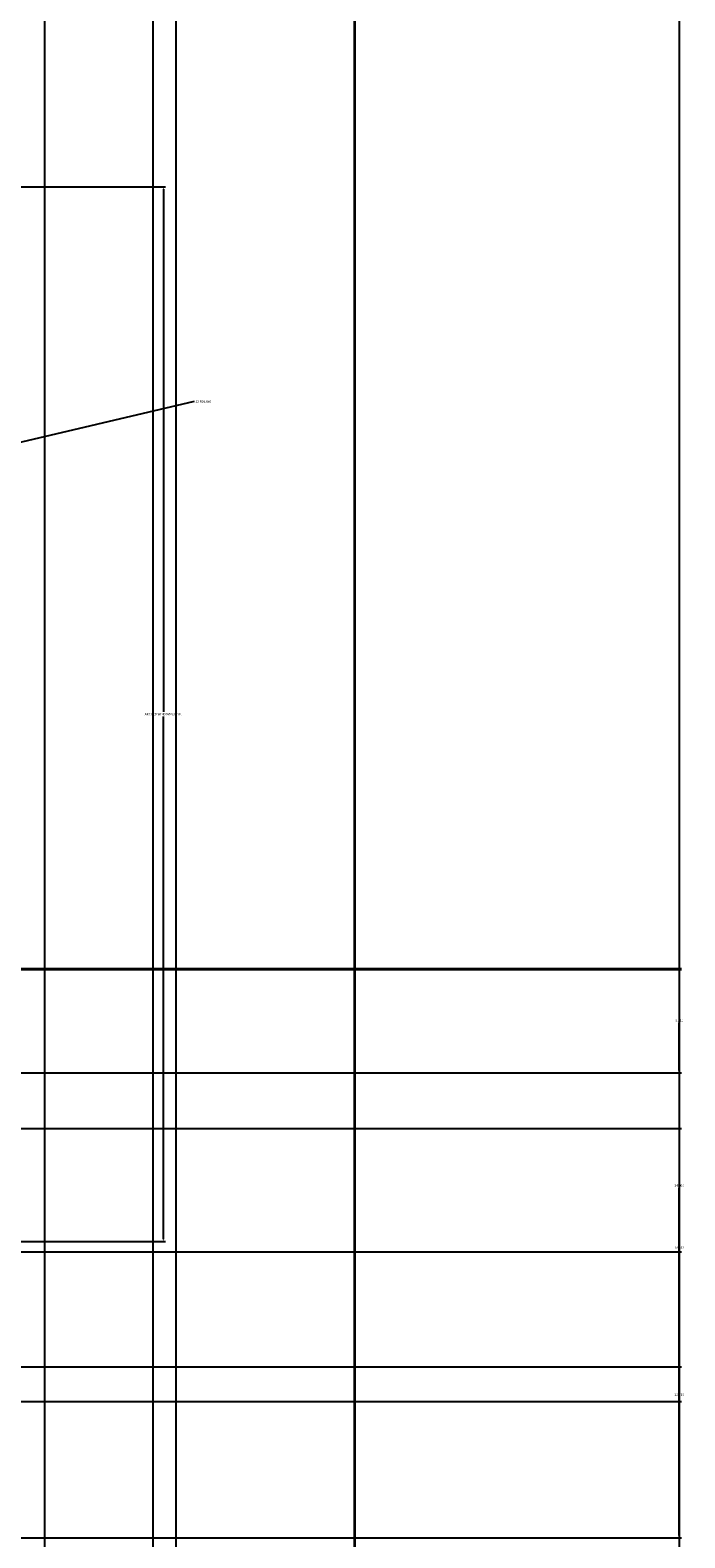
# Model space of a CAD drawing. Units: inches. Extents: x 93 to 565, y 123 to 656.
# Tile 16 of 18: x 513 to 565, y 463 to 582. Entities that reach past the tile are written whole.
import ezdxf

# ---------------------------------------------------------------- set-up
doc = ezdxf.new("R2010")
doc.units = ezdxf.units.IN
doc.header["$MEASUREMENT"] = 0
doc.layers.add('A-ANNO-DIMS', color=2, linetype='Continuous', lineweight=18)
doc.layers.add('A-ELEV', color=7, linetype='Continuous', lineweight=35)
doc.styles.get("Standard").update_dxf_attribs({"font": 'arial.ttf'})
doc.dimstyles.get("Standard").update_dxf_attribs({"dimtxt": 0.18, "dimasz": 0.18, "dimexe": 0.18, "dimexo": 0.0625, "dimgap": 0.09, "dimtad": 0, "dimtih": 1, "dimtoh": 1, "dimdec": 4, "dimzin": 0, "dimdsep": 46, "dimtxsty": 'Standard', "dimcen": 0.09, "dimadec": 0, "dimazin": 0, "dimtfac": 1, "dimtdec": 4, "dimtofl": 0, "dimtmove": 0, "dimatfit": 3, "dimfxl": 1, "dimtolj": 1, "dimtzin": 0, "dimarcsym": 0})

# ---------------------------------------------------------------- blocks, each defined once
blk = doc.blocks.new('*D20')
at = {"layer": 'A-ANNO-DIMS', "color": 0, "lineweight": -2, "transparency": 16777216}
for p, q in [((511.59, 569.37), (524.16, 569.37)), ((523.98, 569.19), (523.98, 528.03)), ((523.98, 486.5), (523.98, 527.66)), ((511.59, 486.32), (524.16, 486.32))]:
    blk.add_line(p, q, dxfattribs=at)
at = {"layer": 'A-ANNO-DIMS', "color": 0, "transparency": 16777216}
for points in [[(523.95, 569.19), (524.01, 569.19), (523.98, 569.37)], [(523.95, 486.5), (524.01, 486.5), (523.98, 486.32)]]:
    blk.add_solid(points, dxfattribs=at)
at = {"layer": 'Defpoints', "color": 0, "transparency": 16777216}
for p in [(511.53, 569.37), (523.98, 569.37), (511.53, 486.32)]:
    blk.add_point(p, dxfattribs=at)
at = {"layer": 'A-ANNO-DIMS', "color": 0, "transparency": 16777216, "insert": (523.98, 527.85), "char_height": 0.18, "attachment_point": 5}
blk.add_mtext('\\A1;ARCHED WINDOW 83 TYP.', dxfattribs=at)
blk = doc.blocks.new('*D26')
at = {"layer": 'A-ANNO-DIMS', "color": 0, "lineweight": -2, "transparency": 16777216}
for p, q in [((119.08, 519.16), (119.08, 656.13)), ((119.26, 655.95), (328.79, 655.95)), ((538.9, 655.95), (329.37, 655.95)), ((539.08, 630.47), (539.08, 656.13))]:
    blk.add_line(p, q, dxfattribs=at)
at = {"layer": 'A-ANNO-DIMS', "color": 0, "transparency": 16777216}
for points in [[(119.26, 655.98), (119.26, 655.92), (119.08, 655.95)], [(538.9, 655.98), (538.9, 655.92), (539.08, 655.95)]]:
    blk.add_solid(points, dxfattribs=at)
at = {"layer": 'Defpoints', "color": 0, "transparency": 16777216}
for p in [(539.08, 655.95), (539.08, 630.4), (119.08, 519.1)]:
    blk.add_point(p, dxfattribs=at)
at = {"layer": 'A-ANNO-DIMS', "color": 0, "transparency": 16777216, "insert": (329.08, 655.95), "char_height": 0.18, "attachment_point": 5}
blk.add_mtext('\\A1;420', dxfattribs=at)
blk = doc.blocks.new('*D30')
at = {"layer": 'A-ANNO-DIMS', "color": 0, "lineweight": -2, "transparency": 16777216}
for p, q in [((437.19, 594.34), (437.19, 134)), ((539.08, 159.67), (539.08, 134)), ((437.37, 134.18), (487.75, 134.18)), ((538.9, 134.18), (488.52, 134.18))]:
    blk.add_line(p, q, dxfattribs=at)
at = {"layer": 'A-ANNO-DIMS', "color": 0, "transparency": 16777216}
for points in [[(437.37, 134.21), (437.37, 134.15), (437.19, 134.18)], [(538.9, 134.21), (538.9, 134.15), (539.08, 134.18)]]:
    blk.add_solid(points, dxfattribs=at)
at = {"layer": 'Defpoints', "color": 0, "transparency": 16777216}
for p in [(437.19, 594.4), (539.08, 159.73), (539.08, 134.18)]:
    blk.add_point(p, dxfattribs=at)
at = {"layer": 'A-ANNO-DIMS', "color": 0, "transparency": 16777216, "insert": (488.13, 134.18), "char_height": 0.18, "attachment_point": 5}
blk.add_mtext('\\A1;101.9', dxfattribs=at)
blk = doc.blocks.new('*D31')
at = {"layer": 'A-ANNO-DIMS', "color": 0, "lineweight": -2, "transparency": 16777216}
for p, q in [((417.87, 630.4), (564.81, 630.4)), ((564.63, 630.22), (564.63, 395.25)), ((564.63, 159.91), (564.63, 394.89)), ((119.14, 159.73), (564.81, 159.73))]:
    blk.add_line(p, q, dxfattribs=at)
at = {"layer": 'A-ANNO-DIMS', "color": 0, "transparency": 16777216}
for points in [[(564.6, 630.22), (564.66, 630.22), (564.63, 630.4)], [(564.6, 159.91), (564.66, 159.91), (564.63, 159.73)]]:
    blk.add_solid(points, dxfattribs=at)
at = {"layer": 'Defpoints', "color": 0, "transparency": 16777216}
for p in [(417.81, 630.4), (564.63, 630.4), (119.08, 159.73)]:
    blk.add_point(p, dxfattribs=at)
at = {"layer": 'A-ANNO-DIMS', "color": 0, "transparency": 16777216, "insert": (564.63, 395.07), "char_height": 0.18, "attachment_point": 5}
blk.add_mtext('\\A1;470.7', dxfattribs=at)
blk = doc.blocks.new('*D73')
at = {"layer": 'A-ANNO-DIMS', "color": 0, "lineweight": -2, "transparency": 16777216}
for p, q in [((437.25, 473.73), (564.81, 473.73)), ((564.63, 473.55), (564.63, 460.91)), ((564.63, 447.91), (564.63, 460.55)), ((437.25, 447.73), (564.81, 447.73))]:
    blk.add_line(p, q, dxfattribs=at)
at = {"layer": 'A-ANNO-DIMS', "color": 0, "transparency": 16777216}
for points in [[(564.6, 473.55), (564.66, 473.55), (564.63, 473.73)], [(564.6, 447.91), (564.66, 447.91), (564.63, 447.73)]]:
    blk.add_solid(points, dxfattribs=at)
at = {"layer": 'Defpoints', "color": 0, "transparency": 16777216}
for p in [(437.19, 473.73), (564.63, 473.73), (437.19, 447.73)]:
    blk.add_point(p, dxfattribs=at)
at = {"layer": 'A-ANNO-DIMS', "color": 0, "transparency": 16777216, "insert": (564.63, 460.73), "char_height": 0.18, "attachment_point": 5}
blk.add_mtext('\\A1;26', dxfattribs=at)
blk = doc.blocks.new('*D74')
at = {"layer": 'A-ANNO-DIMS', "color": 0, "lineweight": -2, "transparency": 16777216}
for p, q in [((437.25, 507.73), (564.81, 507.73)), ((564.63, 507.55), (564.63, 490.91)), ((564.63, 473.91), (564.63, 490.55)), ((437.25, 473.73), (564.81, 473.73))]:
    blk.add_line(p, q, dxfattribs=at)
at = {"layer": 'A-ANNO-DIMS', "color": 0, "transparency": 16777216}
for points in [[(564.6, 507.55), (564.66, 507.55), (564.63, 507.73)], [(564.6, 473.91), (564.66, 473.91), (564.63, 473.73)]]:
    blk.add_solid(points, dxfattribs=at)
at = {"layer": 'Defpoints', "color": 0, "transparency": 16777216}
for p in [(437.19, 507.73), (564.63, 507.73), (437.19, 473.73)]:
    blk.add_point(p, dxfattribs=at)
at = {"layer": 'A-ANNO-DIMS', "color": 0, "transparency": 16777216, "insert": (564.63, 490.73), "char_height": 0.18, "attachment_point": 5}
blk.add_mtext('\\A1;34', dxfattribs=at)
blk = doc.blocks.new('*D77')
at = {"layer": 'A-ANNO-DIMS', "color": 0, "lineweight": -2, "transparency": 16777216}
for p, q in [((399.76, 507.83), (564.81, 507.83)), ((564.63, 507.65), (564.63, 503.9)), ((564.63, 499.79), (564.63, 503.54)), ((375.07, 499.61), (564.81, 499.61))]:
    blk.add_line(p, q, dxfattribs=at)
at = {"layer": 'A-ANNO-DIMS', "color": 0, "transparency": 16777216}
for points in [[(564.6, 507.65), (564.66, 507.65), (564.63, 507.83)], [(564.6, 499.79), (564.66, 499.79), (564.63, 499.61)]]:
    blk.add_solid(points, dxfattribs=at)
at = {"layer": 'Defpoints', "color": 0, "transparency": 16777216}
for p in [(399.69, 507.83), (564.63, 507.83), (375.01, 499.61)]:
    blk.add_point(p, dxfattribs=at)
at = {"layer": 'A-ANNO-DIMS', "color": 0, "transparency": 16777216, "insert": (564.63, 503.72), "char_height": 0.18, "attachment_point": 5}
blk.add_mtext('\\A1;8.221', dxfattribs=at)
blk = doc.blocks.new('*D79')
at = {"layer": 'A-ANNO-DIMS', "color": 0, "lineweight": -2, "transparency": 16777216}
for p, q in [((391.28, 495.22), (564.81, 495.22)), ((564.63, 495.04), (564.63, 486.02)), ((564.63, 476.64), (564.63, 485.66)), ((391.28, 476.46), (564.81, 476.46))]:
    blk.add_line(p, q, dxfattribs=at)
at = {"layer": 'A-ANNO-DIMS', "color": 0, "transparency": 16777216}
for points in [[(564.6, 495.04), (564.66, 495.04), (564.63, 495.22)], [(564.6, 476.64), (564.66, 476.64), (564.63, 476.46)]]:
    blk.add_solid(points, dxfattribs=at)
at = {"layer": 'Defpoints', "color": 0, "transparency": 16777216}
for p in [(391.22, 495.22), (564.63, 495.22), (391.22, 476.46)]:
    blk.add_point(p, dxfattribs=at)
at = {"layer": 'A-ANNO-DIMS', "color": 0, "transparency": 16777216, "insert": (564.63, 485.84), "char_height": 0.18, "attachment_point": 5}
blk.add_mtext('\\A1;18.753', dxfattribs=at)
blk = doc.blocks.new('*D85')
at = {"layer": 'A-ANNO-DIMS', "color": 0, "lineweight": -2, "transparency": 16777216}
for p, q in [((457.46, 485.52), (564.81, 485.52)), ((564.63, 485.34), (564.63, 474.44)), ((564.63, 463.17), (564.63, 474.07)), ((484.92, 462.99), (564.81, 462.99))]:
    blk.add_line(p, q, dxfattribs=at)
at = {"layer": 'A-ANNO-DIMS', "color": 0, "transparency": 16777216}
for points in [[(564.6, 485.34), (564.66, 485.34), (564.63, 485.52)], [(564.6, 463.17), (564.66, 463.17), (564.63, 462.99)]]:
    blk.add_solid(points, dxfattribs=at)
at = {"layer": 'Defpoints', "color": 0, "transparency": 16777216}
for p in [(457.39, 485.52), (564.63, 485.52), (484.86, 462.99)]:
    blk.add_point(p, dxfattribs=at)
at = {"layer": 'A-ANNO-DIMS', "color": 0, "transparency": 16777216, "insert": (564.63, 474.25), "char_height": 0.18, "attachment_point": 5}
blk.add_mtext('\\A1;22.535', dxfattribs=at)
blk = doc.blocks.new('*D92')
at = {"layer": 'A-ANNO-DIMS', "color": 0, "lineweight": -2, "transparency": 16777216}
for p, q in [((523.14, 603.14), (523.14, 134)), ((499.73, 599.75), (499.73, 134)), ((499.91, 134.18), (510.97, 134.18)), ((522.96, 134.18), (511.9, 134.18))]:
    blk.add_line(p, q, dxfattribs=at)
at = {"layer": 'A-ANNO-DIMS', "color": 0, "transparency": 16777216}
for points in [[(499.91, 134.21), (499.91, 134.15), (499.73, 134.18)], [(522.96, 134.21), (522.96, 134.15), (523.14, 134.18)]]:
    blk.add_solid(points, dxfattribs=at)
at = {"layer": 'Defpoints', "color": 0, "transparency": 16777216}
for p in [(523.14, 603.2), (499.73, 599.82), (523.14, 134.18)]:
    blk.add_point(p, dxfattribs=at)
at = {"layer": 'A-ANNO-DIMS', "color": 0, "transparency": 16777216, "insert": (511.44, 134.18), "char_height": 0.18, "attachment_point": 5}
blk.add_mtext('\\A1;23.412', dxfattribs=at)
blk = doc.blocks.new('*D93')
at = {"layer": 'A-ANNO-DIMS', "color": 0, "lineweight": -2, "transparency": 16777216}
for p, q in [((523.14, 603.14), (523.14, 134)), ((539.08, 594.34), (539.08, 134)), ((523.32, 134.18), (530.66, 134.18)), ((538.9, 134.18), (531.57, 134.18))]:
    blk.add_line(p, q, dxfattribs=at)
at = {"layer": 'A-ANNO-DIMS', "color": 0, "transparency": 16777216}
for points in [[(523.32, 134.21), (523.32, 134.15), (523.14, 134.18)], [(538.9, 134.21), (538.9, 134.15), (539.08, 134.18)]]:
    blk.add_solid(points, dxfattribs=at)
at = {"layer": 'Defpoints', "color": 0, "transparency": 16777216}
for p in [(523.14, 603.2), (539.08, 594.4), (539.08, 134.18)]:
    blk.add_point(p, dxfattribs=at)
at = {"layer": 'A-ANNO-DIMS', "color": 0, "transparency": 16777216, "insert": (531.11, 134.18), "char_height": 0.18, "attachment_point": 5}
blk.add_mtext('\\A1;15.938', dxfattribs=at)
blk = doc.blocks.new('*D102')
at = {"layer": 'A-ANNO-DIMS', "color": 0, "lineweight": -2, "transparency": 16777216}
for p, q in [((526.4, 552.46), (511, 548.84)), ((484.77, 542.71), (484.95, 542.71)), ((484.86, 542.62), (484.86, 542.8))]:
    blk.add_line(p, q, dxfattribs=at)
at = {"layer": 'A-ANNO-DIMS', "color": 0, "transparency": 16777216}
blk.add_solid([(510.99, 548.87), (511, 548.81), (510.82, 548.8)], dxfattribs=at)
at = {"layer": 'Defpoints', "color": 0, "transparency": 16777216}
for p in [(510.82, 548.8), (484.86, 542.71)]:
    blk.add_point(p, dxfattribs=at)
at = {"layer": 'A-ANNO-DIMS', "color": 0, "transparency": 16777216, "insert": (527.14, 552.46), "char_height": 0.18, "attachment_point": 5}
blk.add_mtext('\\A1;2X R26.666', dxfattribs=at)
blk = doc.blocks.new('*D105')
at = {"layer": 'A-ANNO-DIMS', "color": 0, "lineweight": -2, "transparency": 16777216}
for p, q in [((119.08, 519.16), (119.08, 656.13)), ((119.26, 655.95), (328.54, 655.95)), ((538.9, 655.95), (329.62, 655.95)), ((539.08, 630.47), (539.08, 656.13))]:
    blk.add_line(p, q, dxfattribs=at)
at = {"layer": 'A-ANNO-DIMS', "color": 0, "transparency": 16777216}
for points in [[(119.26, 655.98), (119.26, 655.92), (119.08, 655.95)], [(538.9, 655.98), (538.9, 655.92), (539.08, 655.95)]]:
    blk.add_solid(points, dxfattribs=at)
at = {"layer": 'Defpoints', "color": 0, "transparency": 16777216}
for p in [(539.08, 655.95), (539.08, 630.4), (119.08, 519.1)]:
    blk.add_point(p, dxfattribs=at)
at = {"layer": 'A-ANNO-DIMS', "color": 0, "transparency": 16777216, "insert": (329.08, 655.95), "char_height": 0.18, "attachment_point": 5}
blk.add_mtext('\\A1;420.000', dxfattribs=at)
blk = doc.blocks.new('*D109')
at = {"layer": 'A-ANNO-DIMS', "color": 0, "lineweight": -2, "transparency": 16777216}
for p, q in [((437.19, 594.34), (437.19, 134)), ((539.08, 159.67), (539.08, 134)), ((437.37, 134.18), (487.63, 134.18)), ((538.9, 134.18), (488.64, 134.18))]:
    blk.add_line(p, q, dxfattribs=at)
at = {"layer": 'A-ANNO-DIMS', "color": 0, "transparency": 16777216}
for points in [[(437.37, 134.21), (437.37, 134.15), (437.19, 134.18)], [(538.9, 134.21), (538.9, 134.15), (539.08, 134.18)]]:
    blk.add_solid(points, dxfattribs=at)
at = {"layer": 'Defpoints', "color": 0, "transparency": 16777216}
for p in [(437.19, 594.4), (539.08, 159.73), (539.08, 134.18)]:
    blk.add_point(p, dxfattribs=at)
at = {"layer": 'A-ANNO-DIMS', "color": 0, "transparency": 16777216, "insert": (488.13, 134.18), "char_height": 0.18, "attachment_point": 5}
blk.add_mtext('\\A1;101.891', dxfattribs=at)
blk = doc.blocks.new('*D110')
at = {"layer": 'A-ANNO-DIMS', "color": 0, "lineweight": -2, "transparency": 16777216}
for p, q in [((417.87, 630.4), (564.81, 630.4)), ((564.63, 630.22), (564.63, 395.25)), ((564.63, 159.91), (564.63, 394.89)), ((119.14, 159.73), (564.81, 159.73))]:
    blk.add_line(p, q, dxfattribs=at)
at = {"layer": 'A-ANNO-DIMS', "color": 0, "transparency": 16777216}
for points in [[(564.6, 630.22), (564.66, 630.22), (564.63, 630.4)], [(564.6, 159.91), (564.66, 159.91), (564.63, 159.73)]]:
    blk.add_solid(points, dxfattribs=at)
at = {"layer": 'Defpoints', "color": 0, "transparency": 16777216}
for p in [(417.81, 630.4), (564.63, 630.4), (119.08, 159.73)]:
    blk.add_point(p, dxfattribs=at)
at = {"layer": 'A-ANNO-DIMS', "color": 0, "transparency": 16777216, "insert": (564.63, 395.07), "char_height": 0.18, "attachment_point": 5}
blk.add_mtext('\\A1;470.673', dxfattribs=at)
blk = doc.blocks.new('*D152')
at = {"layer": 'A-ANNO-DIMS', "color": 0, "lineweight": -2, "transparency": 16777216}
for p, q in [((437.25, 473.73), (564.81, 473.73)), ((564.63, 473.55), (564.63, 460.91)), ((564.63, 447.91), (564.63, 460.55)), ((437.25, 447.73), (564.81, 447.73))]:
    blk.add_line(p, q, dxfattribs=at)
at = {"layer": 'A-ANNO-DIMS', "color": 0, "transparency": 16777216}
for points in [[(564.6, 473.55), (564.66, 473.55), (564.63, 473.73)], [(564.6, 447.91), (564.66, 447.91), (564.63, 447.73)]]:
    blk.add_solid(points, dxfattribs=at)
at = {"layer": 'Defpoints', "color": 0, "transparency": 16777216}
for p in [(437.19, 473.73), (564.63, 473.73), (437.19, 447.73)]:
    blk.add_point(p, dxfattribs=at)
at = {"layer": 'A-ANNO-DIMS', "color": 0, "transparency": 16777216, "insert": (564.63, 460.73), "char_height": 0.18, "attachment_point": 5}
blk.add_mtext('\\A1;26.000', dxfattribs=at)
blk = doc.blocks.new('*D153')
at = {"layer": 'A-ANNO-DIMS', "color": 0, "lineweight": -2, "transparency": 16777216}
for p, q in [((437.25, 507.73), (564.81, 507.73)), ((564.63, 507.55), (564.63, 490.91)), ((564.63, 473.91), (564.63, 490.55)), ((437.25, 473.73), (564.81, 473.73))]:
    blk.add_line(p, q, dxfattribs=at)
at = {"layer": 'A-ANNO-DIMS', "color": 0, "transparency": 16777216}
for points in [[(564.6, 507.55), (564.66, 507.55), (564.63, 507.73)], [(564.6, 473.91), (564.66, 473.91), (564.63, 473.73)]]:
    blk.add_solid(points, dxfattribs=at)
at = {"layer": 'Defpoints', "color": 0, "transparency": 16777216}
for p in [(437.19, 507.73), (564.63, 507.73), (437.19, 473.73)]:
    blk.add_point(p, dxfattribs=at)
at = {"layer": 'A-ANNO-DIMS', "color": 0, "transparency": 16777216, "insert": (564.63, 490.73), "char_height": 0.18, "attachment_point": 5}
blk.add_mtext('\\A1;34.000', dxfattribs=at)
blk = doc.blocks.new('*D156')
at = {"layer": 'A-ANNO-DIMS', "color": 0, "lineweight": -2, "transparency": 16777216}
for p, q in [((399.76, 507.83), (564.81, 507.83)), ((564.63, 507.65), (564.63, 503.9)), ((564.63, 499.79), (564.63, 503.54)), ((375.07, 499.61), (564.81, 499.61))]:
    blk.add_line(p, q, dxfattribs=at)
at = {"layer": 'A-ANNO-DIMS', "color": 0, "transparency": 16777216}
for points in [[(564.6, 507.65), (564.66, 507.65), (564.63, 507.83)], [(564.6, 499.79), (564.66, 499.79), (564.63, 499.61)]]:
    blk.add_solid(points, dxfattribs=at)
at = {"layer": 'Defpoints', "color": 0, "transparency": 16777216}
for p in [(399.69, 507.83), (564.63, 507.83), (375.01, 499.61)]:
    blk.add_point(p, dxfattribs=at)
at = {"layer": 'A-ANNO-DIMS', "color": 0, "transparency": 16777216, "insert": (564.63, 503.72), "char_height": 0.18, "attachment_point": 5}
blk.add_mtext('\\A1;8.221', dxfattribs=at)
blk = doc.blocks.new('*D158')
at = {"layer": 'A-ANNO-DIMS', "color": 0, "lineweight": -2, "transparency": 16777216}
for p, q in [((391.28, 495.22), (564.81, 495.22)), ((564.63, 495.04), (564.63, 486.02)), ((564.63, 476.64), (564.63, 485.66)), ((391.28, 476.46), (564.81, 476.46))]:
    blk.add_line(p, q, dxfattribs=at)
at = {"layer": 'A-ANNO-DIMS', "color": 0, "transparency": 16777216}
for points in [[(564.6, 495.04), (564.66, 495.04), (564.63, 495.22)], [(564.6, 476.64), (564.66, 476.64), (564.63, 476.46)]]:
    blk.add_solid(points, dxfattribs=at)
at = {"layer": 'Defpoints', "color": 0, "transparency": 16777216}
for p in [(391.22, 495.22), (564.63, 495.22), (391.22, 476.46)]:
    blk.add_point(p, dxfattribs=at)
at = {"layer": 'A-ANNO-DIMS', "color": 0, "transparency": 16777216, "insert": (564.63, 485.84), "char_height": 0.18, "attachment_point": 5}
blk.add_mtext('\\A1;18.753', dxfattribs=at)
blk = doc.blocks.new('*D164')
at = {"layer": 'A-ANNO-DIMS', "color": 0, "lineweight": -2, "transparency": 16777216}
for p, q in [((457.46, 485.52), (564.81, 485.52)), ((564.63, 485.34), (564.63, 474.44)), ((564.63, 463.17), (564.63, 474.07)), ((484.92, 462.99), (564.81, 462.99))]:
    blk.add_line(p, q, dxfattribs=at)
at = {"layer": 'A-ANNO-DIMS', "color": 0, "transparency": 16777216}
for points in [[(564.6, 485.34), (564.66, 485.34), (564.63, 485.52)], [(564.6, 463.17), (564.66, 463.17), (564.63, 462.99)]]:
    blk.add_solid(points, dxfattribs=at)
at = {"layer": 'Defpoints', "color": 0, "transparency": 16777216}
for p in [(457.39, 485.52), (564.63, 485.52), (484.86, 462.99)]:
    blk.add_point(p, dxfattribs=at)
at = {"layer": 'A-ANNO-DIMS', "color": 0, "transparency": 16777216, "insert": (564.63, 474.25), "char_height": 0.18, "attachment_point": 5}
blk.add_mtext('\\A1;22.535', dxfattribs=at)
blk = doc.blocks.new('*D171')
at = {"layer": 'A-ANNO-DIMS', "color": 0, "lineweight": -2, "transparency": 16777216}
for p, q in [((523.14, 603.14), (523.14, 134)), ((499.73, 599.75), (499.73, 134)), ((499.91, 134.18), (510.97, 134.18)), ((522.96, 134.18), (511.9, 134.18))]:
    blk.add_line(p, q, dxfattribs=at)
at = {"layer": 'A-ANNO-DIMS', "color": 0, "transparency": 16777216}
for points in [[(499.91, 134.21), (499.91, 134.15), (499.73, 134.18)], [(522.96, 134.21), (522.96, 134.15), (523.14, 134.18)]]:
    blk.add_solid(points, dxfattribs=at)
at = {"layer": 'Defpoints', "color": 0, "transparency": 16777216}
for p in [(523.14, 603.2), (499.73, 599.82), (523.14, 134.18)]:
    blk.add_point(p, dxfattribs=at)
at = {"layer": 'A-ANNO-DIMS', "color": 0, "transparency": 16777216, "insert": (511.44, 134.18), "char_height": 0.18, "attachment_point": 5}
blk.add_mtext('\\A1;23.412', dxfattribs=at)
blk = doc.blocks.new('*D172')
at = {"layer": 'A-ANNO-DIMS', "color": 0, "lineweight": -2, "transparency": 16777216}
for p, q in [((523.14, 603.14), (523.14, 134)), ((539.08, 594.34), (539.08, 134)), ((523.32, 134.18), (530.66, 134.18)), ((538.9, 134.18), (531.57, 134.18))]:
    blk.add_line(p, q, dxfattribs=at)
at = {"layer": 'A-ANNO-DIMS', "color": 0, "transparency": 16777216}
for points in [[(523.32, 134.21), (523.32, 134.15), (523.14, 134.18)], [(538.9, 134.21), (538.9, 134.15), (539.08, 134.18)]]:
    blk.add_solid(points, dxfattribs=at)
at = {"layer": 'Defpoints', "color": 0, "transparency": 16777216}
for p in [(523.14, 603.2), (539.08, 594.4), (539.08, 134.18)]:
    blk.add_point(p, dxfattribs=at)
at = {"layer": 'A-ANNO-DIMS', "color": 0, "transparency": 16777216, "insert": (531.11, 134.18), "char_height": 0.18, "attachment_point": 5}
blk.add_mtext('\\A1;15.938', dxfattribs=at)
blk = doc.blocks.new('*D185')
at = {"layer": 'A-ANNO-DIMS', "color": 0, "lineweight": -2, "transparency": 16777216}
for p, q in [((514.64, 358.44), (514.64, 656.13)), ((514.82, 655.95), (519.36, 655.95)), ((524.81, 655.95), (520.27, 655.95)), ((524.99, 363.79), (524.99, 656.13))]:
    blk.add_line(p, q, dxfattribs=at)
at = {"layer": 'A-ANNO-DIMS', "color": 0, "transparency": 16777216}
for points in [[(514.82, 655.98), (514.82, 655.92), (514.64, 655.95)], [(524.81, 655.98), (524.81, 655.92), (524.99, 655.95)]]:
    blk.add_solid(points, dxfattribs=at)
at = {"layer": 'Defpoints', "color": 0, "transparency": 16777216}
for p in [(524.99, 655.95), (524.99, 363.73), (514.64, 358.37)]:
    blk.add_point(p, dxfattribs=at)
at = {"layer": 'A-ANNO-DIMS', "color": 0, "transparency": 16777216, "insert": (519.81, 655.95), "char_height": 0.18, "attachment_point": 5}
blk.add_mtext('\\A1;10.344', dxfattribs=at)
blk = doc.blocks.new('*D186')
at = {"layer": 'A-ANNO-DIMS', "color": 0, "lineweight": -2, "transparency": 16777216}
for p, q in [((524.99, 363.79), (524.99, 656.13)), ((525.17, 655.95), (531.58, 655.95)), ((538.9, 655.95), (532.49, 655.95)), ((539.08, 363.79), (539.08, 656.13))]:
    blk.add_line(p, q, dxfattribs=at)
at = {"layer": 'A-ANNO-DIMS', "color": 0, "transparency": 16777216}
for points in [[(525.17, 655.98), (525.17, 655.92), (524.99, 655.95)], [(538.9, 655.98), (538.9, 655.92), (539.08, 655.95)]]:
    blk.add_solid(points, dxfattribs=at)
at = {"layer": 'Defpoints', "color": 0, "transparency": 16777216}
for p in [(539.08, 655.95), (524.99, 363.73), (539.08, 363.73)]:
    blk.add_point(p, dxfattribs=at)
at = {"layer": 'A-ANNO-DIMS', "color": 0, "transparency": 16777216, "insert": (532.03, 655.95), "char_height": 0.18, "attachment_point": 5}
blk.add_mtext('\\A1;14.093', dxfattribs=at)

msp = doc.modelspace()

# ---------------------------------------------------------------- linework, layer by layer
at = {"layer": 'A-ELEV'}
msp.add_line((539.0794, 363.7323), (539.0794, 594.4048), dxfattribs=at)

# ---------------------------------------------------------------- dimensions: what is measured, and where the dimension line sits
at = {"layer": 'A-ANNO-DIMS'}
for base, p1, p2, override, picture, middle in [((539.0794, 655.9548), (119.0794, 519.0999), (539.0794, 630.4048), {"dimdec": 0, "dimlfac": 1, "dimrnd": 0, "dimzin": 0, "dimdsep": 46, "dimlunit": 2}, '*D26', (329.0794, 655.9548)), ((539.0794, 655.9548), (119.0794, 519.0999), (539.0794, 630.4048), {"dimdec": 3, "dimlfac": 1, "dimrnd": 0, "dimzin": 0, "dimdsep": 46, "dimlunit": 2}, '*D105', (329.0794, 655.9548)), ((524.9864, 655.9548), (514.6424, 358.3735), (524.9864, 363.7323), {"dimdec": 3, "dimlfac": 1, "dimrnd": 0, "dimzin": 0, "dimdsep": 46, "dimlunit": 2}, '*D185', (519.8144, 655.9548)), ((539.0794, 655.9548), (524.9864, 363.7323), (539.0794, 363.7323), {"dimdec": 3, "dimlfac": 1, "dimrnd": 0, "dimzin": 0, "dimdsep": 46, "dimlunit": 2}, '*D186', (532.0329, 655.9548)), ((523.1415, 134.1823), (499.7291, 599.8171), (523.1415, 603.1979), {"dimdec": 3, "dimlfac": 1, "dimrnd": 0, "dimzin": 0, "dimdsep": 46, "dimlunit": 2}, '*D92', (511.4353, 134.1823)), ((523.1415, 134.1823), (499.7291, 599.8171), (523.1415, 603.1979), {"dimdec": 3, "dimlfac": 1, "dimrnd": 0, "dimzin": 0, "dimdsep": 46, "dimlunit": 2}, '*D171', (511.4353, 134.1823)), ((539.0794, 134.1823), (523.1415, 603.1979), (539.0794, 594.4048), {"dimdec": 3, "dimlfac": 1, "dimrnd": 0, "dimzin": 0, "dimdsep": 46, "dimlunit": 2}, '*D93', (531.1104, 134.1823)), ((539.0794, 134.1823), (523.1415, 603.1979), (539.0794, 594.4048), {"dimdec": 3, "dimlfac": 1, "dimrnd": 0, "dimzin": 0, "dimdsep": 46, "dimlunit": 2}, '*D172', (531.1104, 134.1823)), ((539.0794, 134.1823), (437.1885, 594.4048), (539.0794, 159.7323), {"dimdec": 1, "dimlfac": 1, "dimrnd": 0, "dimzin": 0, "dimdsep": 46, "dimlunit": 2}, '*D30', (488.1339, 134.1823)), ((539.0794, 134.1823), (437.1885, 594.4048), (539.0794, 159.7323), {"dimdec": 3, "dimlfac": 1, "dimrnd": 0, "dimzin": 0, "dimdsep": 46, "dimlunit": 2}, '*D109', (488.1339, 134.1823))]:
    dim = msp.add_linear_dim(base=base, p1=p1, p2=p2, dimstyle='Standard', override=override, dxfattribs=at)
    dim.commit()
    dim.dimension.update_dxf_attribs({"geometry": picture, "text_midpoint": middle})
for base, p1, p2, override, picture, middle in [((564.6294, 630.4048), (119.0794, 159.7323), (417.8097, 630.4048), {"dimdec": 1, "dimlfac": 1, "dimrnd": 0, "dimzin": 0, "dimdsep": 46, "dimlunit": 2}, '*D31', (564.6294, 395.0685)), ((564.62936, 630.40478), (119.07936, 159.73225), (417.80971, 630.40477), {"dimdec": 3, "dimlfac": 1, "dimrnd": 0, "dimzin": 0, "dimdsep": 46, "dimlunit": 2}, '*D110', (564.62936, 395.06851)), ((564.6294, 507.8299), (375.0121, 499.609), (399.6946, 507.8299), {"dimdec": 3, "dimlfac": 1, "dimrnd": 0, "dimzin": 0, "dimdsep": 46, "dimlunit": 2}, '*D77', (564.6294, 503.7194)), ((564.6294, 507.8299), (375.0121, 499.609), (399.6946, 507.8299), {"dimdec": 3, "dimlfac": 1, "dimrnd": 0, "dimzin": 0, "dimdsep": 46, "dimlunit": 2}, '*D156', (564.6294, 503.7194)), ((564.6294, 507.7323), (437.1885, 473.7323), (437.1885, 507.7323), {"dimdec": 0, "dimlfac": 1, "dimrnd": 0, "dimzin": 0, "dimdsep": 46, "dimlunit": 2}, '*D74', (564.6294, 490.7323)), ((564.6294, 507.7323), (437.1885, 473.7323), (437.1885, 507.7323), {"dimdec": 3, "dimlfac": 1, "dimrnd": 0, "dimzin": 0, "dimdsep": 46, "dimlunit": 2}, '*D153', (564.6294, 490.7323)), ((564.6294, 495.2171), (391.222, 476.4637), (391.222, 495.2171), {"dimdec": 3, "dimlfac": 1, "dimrnd": 0, "dimzin": 0, "dimdsep": 46, "dimlunit": 2}, '*D79', (564.6294, 485.8404)), ((564.6294, 495.2171), (391.222, 476.4637), (391.222, 495.2171), {"dimdec": 3, "dimlfac": 1, "dimrnd": 0, "dimzin": 0, "dimdsep": 46, "dimlunit": 2}, '*D158', (564.6294, 485.8404)), ((564.6294, 485.5222), (484.8595, 462.9876), (457.3933, 485.5222), {"dimdec": 3, "dimlfac": 1, "dimrnd": 0, "dimzin": 0, "dimdsep": 46, "dimlunit": 2}, '*D85', (564.6294, 474.2549)), ((564.6294, 485.5222), (484.8595, 462.9876), (457.3933, 485.5222), {"dimdec": 3, "dimlfac": 1, "dimrnd": 0, "dimzin": 0, "dimdsep": 46, "dimlunit": 2}, '*D164', (564.6294, 474.2549)), ((564.6294, 473.7323), (437.1885, 447.7323), (437.1885, 473.7323), {"dimdec": 0, "dimlfac": 1, "dimrnd": 0, "dimzin": 0, "dimdsep": 46, "dimlunit": 2}, '*D73', (564.6294, 460.7323)), ((564.6294, 473.7323), (437.1885, 447.7323), (437.1885, 473.7323), {"dimdec": 3, "dimlfac": 1, "dimrnd": 0, "dimzin": 0, "dimdsep": 46, "dimlunit": 2}, '*D152', (564.6294, 460.7323))]:
    dim = msp.add_linear_dim(base=base, p1=p1, p2=p2, angle=90, dimstyle='Standard', override=override, dxfattribs=at)
    dim.commit()
    dim.dimension.update_dxf_attribs({"geometry": picture, "text_midpoint": middle})
dim = msp.add_linear_dim(base=(523.9832, 569.3726), p1=(511.5257, 486.3222), p2=(511.5257, 569.3726), angle=90, text='ARCHED WINDOW <> TYP.', dimstyle='Standard', override={"dimdec": 0, "dimrnd": 0, "dimzin": 0, "dimlunit": 2}, dxfattribs=at)
dim.commit()
dim.dimension.update_dxf_attribs({"geometry": '*D20', "text_midpoint": (523.9832, 527.8474)})
dim = msp.add_radius_dim(center=(484.8595, 542.7064), mpoint=(510.8201, 548.8), text='2X <>', dimstyle='Standard', override={"dimdec": 3, "dimlfac": 1, "dimrnd": 0, "dimzin": 0, "dimdsep": 46, "dimlunit": 2}, dxfattribs=at)
dim.commit()
dim.dimension.update_dxf_attribs({"geometry": '*D102', "text_midpoint": (526.3965, 552.4562), "dimtype": 164})

doc.saveas('drawing.dxf')
